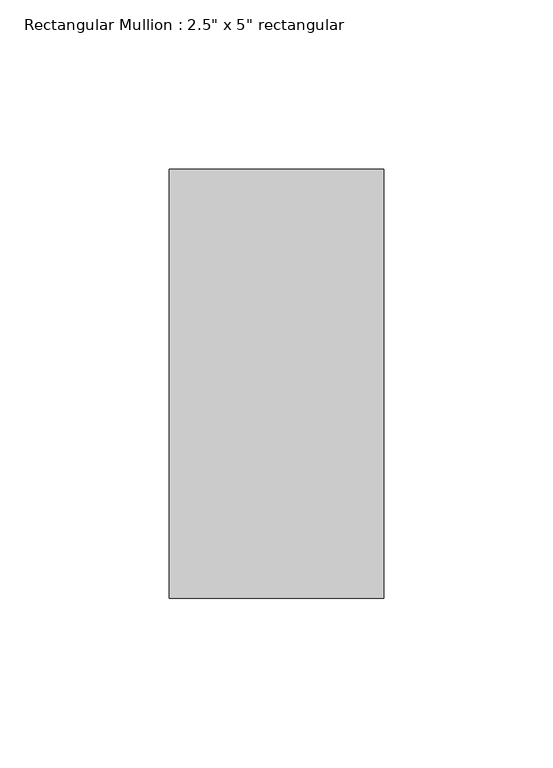
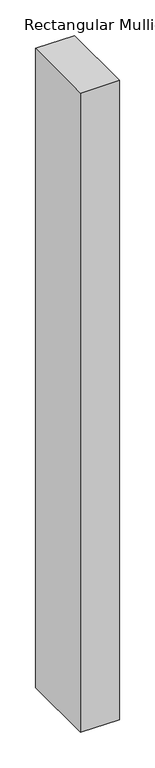
"""IFC4 building model written with IfcOpenShell, lengths in millimetres: member geometry."""

from ifc_helpers import new_model, si_unit, frame, origin, place, context, project, spatial, polyline, outline, extrude, source, transform, mapped, element, save


def member_11eb1482(model_context):
    return source(origin(), model_context, "Body", "SweptSolid", [
        extrude(outline(polyline([(0.0, 63.5), (0.0, -63.5), (-63.5, -63.5), (-63.5, 63.5), (0.0, 63.5)])), frame((0.0, 0.0, -1098.5500002), z_axis=(0.0, 0.0, 1.0), x_axis=(1.0, 0.0, 0.0)), (0.0, 0.0, 1.0), 1098.5500002),
    ])


if __name__ == "__main__":
    model = new_model("IFC4")
    model_context = context("Model", 3, world=origin())
    ifc_project = project(units=[si_unit("LENGTHUNIT", "METRE", prefix="MILLI")], contexts=[model_context])
    site = spatial("IfcSite", under=ifc_project)
    building = spatial("IfcBuilding", under=site)
    placement = place(None, origin())
    member_shape = member_11eb1482(model_context)
    element("IfcMember", 1, ObjectType="Rectangular Mullion : 2.5\" x 5\" rectangular", at=placement, inside=building, context=model_context, shape_type="MappedRepresentation", body=[
        mapped(member_shape, transform((0.0, 0.0, 0.0), x_axis=(1.0, 0.0, 0.0), y_axis=(0.0, 1.0, 0.0), z_axis=(0.0, 0.0, 1.0))),
    ])
    save(model, "model.ifc")

# Revit data of these elements
# Type "Rectangular Mullion : 2.5\" x 5\" rectangular"
#   built-in parameter 1007304 = 0.416667 (stored number, unit not read)
#   built-in parameter 1007301 = 0.104167 (stored number, unit not read)
#   built-in parameter 1007300 = 0.104167 (stored number, unit not read)
# Element 1 (IfcMember, "Rectangular Mullion : 2.5\" x 5\" rectangular")
#   Materials on its faces: "Aluminum"
# Materials
#   "Aluminum": class "Metal", colour RGB 247 247 247, transparency 0, Description = "Aluminum 6061", Cost = 0
